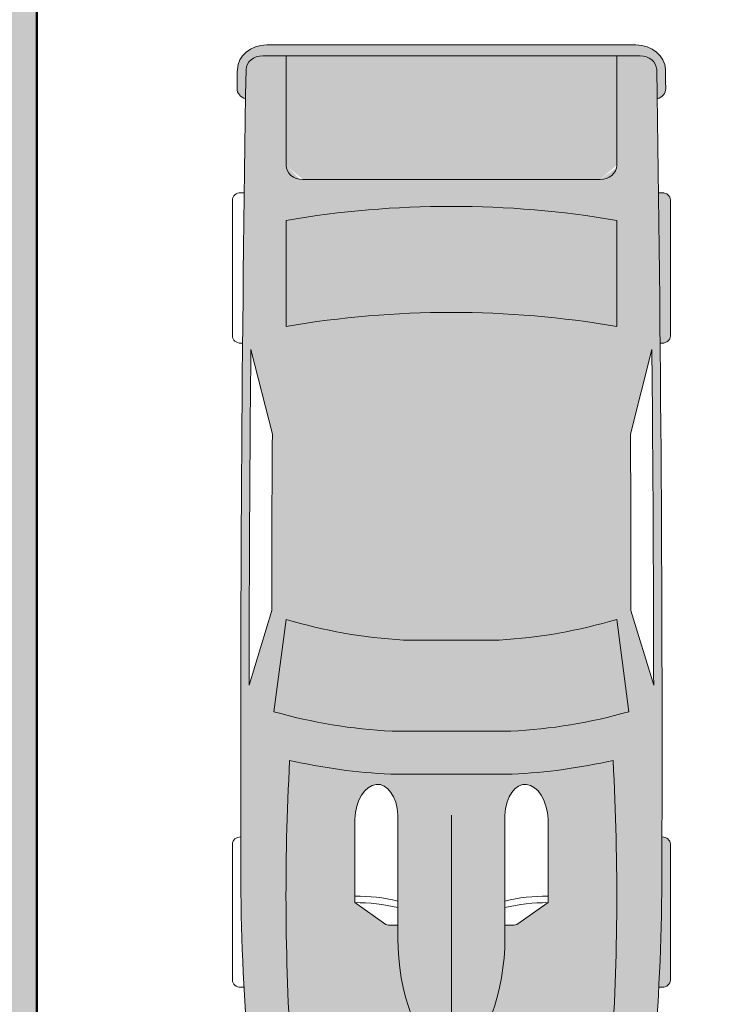
# Model space of a CAD drawing. Units: inches. Extents: x 2419 to 2878, y 1068 to 1713.
# Tile 1 of 20: x 2478 to 2574, y 1153 to 1286. Entities that reach past the tile are written whole.
import ezdxf

# ---------------------------------------------------------------- set-up
doc = ezdxf.new("R2010")
doc.units = ezdxf.units.IN
for name, color, linetype, lineweight in [('A-ANNO-DIMS', 2, 'Continuous', 18), ('A-FLOR-PRKG', 8, 'Continuous', 13), ('A-FLOR-PRKG-PATT', 1, 'Continuous', 13), ('A-FURN-PATT', 254, 'Continuous', 13), ('A-WALL', 7, 'Continuous', 50)]:
    doc.layers.add(name, color=color, linetype=linetype, lineweight=lineweight)
doc.layers.add('A-WALL-PATT', color=18, linetype='Continuous', lineweight=13, true_color=0x000000)
doc.styles.get("Standard").update_dxf_attribs({"font": 'arial.ttf'})
doc.dimstyles.new('ISO-25', dxfattribs={"dimtxt": 12.5, "dimasz": 2.5, "dimexe": 1.25, "dimexo": 0.625, "dimtad": 1, "dimdec": 0, "dimlunit": 4, "dimtxsty": 'Standard', "dimblk": 'ARCHTICK', "dimcen": 2.5, "dimse1": 1, "dimse2": 1, "dimclrd": 4, "dimadec": 0, "dimazin": 0, "dimtfac": 1, "dimtdec": 0, "dimtmove": 0, "dimatfit": 3, "dimfxl": 1, "dimarcsym": 0})

# ---------------------------------------------------------------- blocks, each defined once
blk = doc.blocks.new('*U7')
for p, q in [((46.55368679439944, 38.88847654282876), (22.35054758993934, 38.88847654282876)), ((136.6978032355602, 38.88847654282876), (160.90094244002, 38.88847654282867)), ((21.10406751471477, 37.40863046792069), (21.10406751471477, 36.83230215753705)), ((47.80016686962392, 37.39011648242055), (47.80016686962392, 37.40863046792069)), ((135.4513231603356, 37.07354110333037), (135.4513231603356, 37.40863046792069)), ((162.1474225152445, 37.40863046792049), (162.1474225152445, 36.77402019194128)), ((87.98532186932616, 31.87120872459877), (74.75900729854769, 35.92175679182955)), ((134.313356548143, 35.6043097713567), (119.2882629232503, 31.77757799177584)), ((186.4728846989705, -33.49860931502491), (186.4728846989718, 33.49860931502465)), ((70.0302824853563, 31.53613089391356), (86.40615155322342, 29.35124891408057)), ((188.3990091454065, -32.75868627757393), (188.3990091454077, 32.75868627757058)), ((138.4228833961707, 29.35124891408074), (157.2465674415997, 29.35124891408074)), ((186.4728846989718, 29.35124891408083), (167.0083537481071, 29.35124891408083)), ((164.515393597658, 26.39155676426461), (164.5153935976578, -26.39155676426503)), ((32.26591480791686, 11.62530558863241), (36.12873726252356, 17.16961494239206)), ((36.12873726252356, 17.16961494239206), (50.93891189819171, 17.16961494239206)), ((32.12291633764599, 9.505833383620029), (32.12291633764599, 11.15369945057711)), ((58.9167604809788, -10.77488335095668), (58.9167604809788, 10.77488335095617)), ((66.55009204259746, -10.5288681329018), (66.55009204259746, 10.52886813290129)), ((186.4728846989718, -10.5288681329018), (186.4728846989718, 10.52886813290129)), ((29.77279020470884, 9.505833383620029), (51.68362801571248, 9.505833383620029)), ((82.73706193978568, 8.496039918672748), (82.73706193978568, -8.49603991867258)), ((-4.43e-14, -2.558e-13), (51.68362801571248, -2.558e-13)), ((29.77279020470884, -9.50583338362054), (51.68362801571248, -9.50583338362054)), ((32.12291633764599, -9.50583338362054), (32.12291633764599, -11.15369945057762)), ((32.26591480791686, -11.62530558863292), (36.12873726252356, -17.16961494239257)), ((36.12873726252356, -17.16961494239257), (50.93891189819171, -17.16961494239257)), ((86.40615155322318, -29.35124891408145), (70.03028248535594, -31.53613089391442)), ((157.2465674415997, -29.35124891408117), (138.4228833961707, -29.35124891408126)), ((167.008353748107, -29.35124891408126), (186.4728846989707, -29.35124891408108)), ((87.98532186932607, -31.87120872459903), (74.7590072985476, -35.92175679182964)), ((134.3133565481428, -35.60430977135721), (119.2882629232503, -31.77757799177618)), ((21.10406751471477, -37.4086304679212), (21.10406751471477, -36.83230215753756)), ((47.80016686962392, -37.39011648242107), (47.80016686962392, -37.4086304679212)), ((135.4513231603355, -37.07354110333088), (135.4513231603355, -37.4086304679212)), ((162.1474225152445, -37.408630467921), (162.1474225152445, -36.77402019194179)), ((46.55368679439944, -38.88847654282927), (22.35054758993934, -38.88847654282927)), ((136.6978032355602, -38.88847654282927), (160.9009424400199, -38.88847654282918))]:
    blk.add_line(p, q)
for centre, major_axis, ratio, start_param, end_param in [((22.35054758993934, 37.40863046792072), (2.08e-14, -1.479846074908118), 0.842303869543976, 3.141592653589776, 4.712388980384677), ((46.55368679439944, 37.40863046792072), (2.2e-14, 1.479846074908118), 0.8423038695439758, -1.570796326794884, 1.73e-14), ((136.6978032355602, 37.40863046792072), (2.357e-13, -1.479846074908118), 0.842303869543976, 3.141592653589603, 4.712388980384554), ((160.90094244002, 37.40863046792052), (5.59e-14, 1.479846074908118), 0.842303869543976, -1.570796326794865, 4.44e-14), ((41.19115208863305, -490.8631038926156), (1.294e-13, 528.2339998381949), 0.8423038695439741, 0.0028100083536837, 0.0755983031096952), ((64.48199294511879, -10555.61767587835), (1.907644e-10, 10593.02630634627), 0.842303869543847, -0.0133969486112073, 0.0027970409639888), ((180.6280394947615, 35.8381667808375), (7.4e-14, 2.219769112362114), 0.8423038695439693, -0.0130174256259048, 1.249894140392862), ((64.48199294754608, -10556.35759891604), (1.349839377e-06, 10595.3130398087), 0.8423038681351469, -0.0133969484821159, -0.0130174254969711), ((183.9799245485216, 32.75868627756583), (8.56e-14, -5.246425615115243), 0.8423038695439737, 1.570796326795794, 3.128195704978164), ((64.4819929449925, -10555.61767590795), (1.9177683e-09, -10591.54646030096), 0.8423038695482963, 3.133765086725325, 3.140440689641252), ((183.9799245485226, 33.49860931502124), (3e-16, -2.959692149816168), 0.8423038695439952, 1.570796326796048, 3.128195704978389), ((135.2911776514449, 5.387441675478555), (2.2715e-12, 81.77258453065997), 0.8423038695439563, 1.245306111696802, 1.507880129813836), ((95.78879860270445, -3666.353346297651), (1.949864e-10, -3698.236159209632), 0.8423038695446962, 3.134048706297306, 3.14409775411291), ((37.47375371777758, -593.9621830607928), (6.21e-14, -623.32820996736), 0.8423038695439826, 3.09604606856106, 3.200911180495224), ((134.4003789125686, 5.387441675477674), (4.276e-13, -89.7774543484738), 0.84230386954398, 4.44948196380473, 4.652344057257214), ((149.595361812917, 2.799442537139299), (8.561e-13, -79.57966406425402), 0.842303869543983, 4.372215489277867, 4.640744122441986), ((17.08207736189386, -1.421e-13), (6.87e-14, 147.0179238898305), 0.8423038695439764, 4.511394369635731, 4.913383591133647), ((35.90576140732288, -1.421e-13), (6.87e-14, 147.0179238898305), 0.8423038695439764, 4.511394369635731, 4.913383591133647), ((167.0083537481071, 26.39155676426464), (1.394e-13, 2.959692149816236), 0.842303869543976, 5.55e-14, 1.57079632679492), ((13.03653510440275, 17.00972444508943), (1.2303e-12, 27.41599049210566), 0.8423038695439277, 4.435146050259648, 4.718221029521873), ((14.20086229321332, 17.00972444508943), (1.2303e-12, 27.41599049210566), 0.8423038695439277, 4.435146050259648, 4.718221029521873), ((50.7902773840875, 13.33772416300607), (6.340077547122382, -0.356608581037027), 0.6038335755719145, -1.39555193967809, 1.581314658479915), ((32.74615637525823, 11.15369945057713), (1.313e-13, 0.7399230374541176), 0.8423038695439091, 0.8797135699495516, 1.570796326795045), ((29.77279020470884, -46.66302566589627), (5.12e-14, 56.16885904951626), 0.842303869543976, 7e-16, 0.5903187773915901), ((29.77279020470884, 46.66302566589578), (4.004e-13, 56.16885904951626), 0.8423038695439734, 2.55127387619821, 3.141592653589801), ((149.5953618129329, -2.799442537137565), (4.0897e-12, -79.57966406427697), 0.8423038695439419, -1.499151468852248, -1.230622835688196), ((13.03653510440275, -17.00972444508983), (1.2568e-12, -27.41599049210552), 0.8423038695439318, 1.564964277657711, 1.848039256919935), ((14.20086229321332, -17.00972444508983), (1.2568e-12, -27.41599049210552), 0.8423038695439318, 1.564964277657711, 1.848039256919935), ((32.74615637525823, -11.1536994505777), (1.3e-13, -0.7399230374541176), 0.8423038695439093, 4.712388980384541, 5.403471737230034), ((134.4003789125684, -5.387441675478584), (4.2949e-12, -89.77745434847827), 0.8423038695439354, -1.510751403667474, -1.307889310215002), ((135.2911776514465, -5.387441675480715), (3.2038e-12, -81.77258453066244), 0.8423038695439492, -1.50788012981387, -1.245306111696839), ((167.008353748107, -26.39155676426503), (1.02e-14, -2.959692149816192), 0.8423038695439885, 4.712388980384686, 6.283185307179581), ((37.47375371777847, 593.9621830607904), (1.1693e-12, -623.3282099673584), 0.8423038695439528, -0.0593185269054384, 0.0455465850287298), ((95.78879860271888, 3666.35334629765), (1.637818e-10, -3698.236159209629), 0.8423038695447546, -0.0025051005232382, 0.007543947292366), ((183.9799245485177, -32.7586862775633), (2.428e-13, -5.246425615118353), 0.8423038695439808, 0.0133969486110846, 1.570796326792831), ((183.9799245485216, -33.4986093150211), (9.3e-15, 2.959692149816141), 0.8423038695439732, 3.154989602201626, 4.71238898038339), ((41.19115208863322, 490.8631038926152), (1.37757e-11, -528.2339998381949), 0.8423038695440652, -0.0755983031097181, -0.0028100083537155), ((64.48199294495228, 10555.61767590795), (6.117947e-10, 10593.02630637587), 0.8423038695458146, 3.138795612625926, 3.154989602201039), ((64.48199294503607, 10555.61767590793), (1.6049794e-09, -10591.54646030094), 0.8423038695397146, 0.0011519639481523, 0.0078275668641468), ((180.6280394947581, -35.83816678083949), (2.274e-13, -2.219769112363032), 0.8423038695439803, -1.249894138785958, 0.0130174256254374), ((22.35054758993934, -37.40863046792117), (2.2e-14, 1.479846074908118), 0.8423038695439758, 1.570796326794908, 3.14159265358981), ((46.55368679439944, -37.40863046792117), (2.08e-14, -1.479846074908118), 0.842303869543976, -1.69e-14, 1.570796326794884), ((136.6978032355602, -37.40863046792109), (1.56e-14, -1.479846074908162), 0.8423038695440105, -1.570796326794875, -1.27e-14), ((160.9009424400199, -37.408630467921), (1.969e-13, 1.479846074908162), 0.8423038695440109, 3.141592653589951, 4.712388980384771), ((64.48199294197605, 10556.3575989598), (9.365289701e-07, 10595.31303985772), 0.8423038705260315, 3.154610079306566, 3.154989602290631)]:
    blk.add_ellipse(centre, major_axis=major_axis, ratio=ratio, start_param=start_param, end_param=end_param)
at = {"extrusion": (0, 0, -1)}
blk.add_ellipse((50.7902773840875, -13.33772416300655), major_axis=(6.340077547122382, 0.3566085810370246), ratio=0.6038335755719145, start_param=-1.39555193967809, end_param=1.581314658479915, dxfattribs=at)
blk = doc.blocks.new('_ArchTick')
at = {"color": 0, "linetype": 'ByBlock', "const_width": 0.15}
blk.add_lwpolyline([(-0.5, -0.5), (0.5, 0.5)], dxfattribs=at)
blk = doc.blocks.new('*D38')
at = {"layer": 'A-ANNO-DIMS', "color": 4, "lineweight": -2, "transparency": 16777216}
for p, q in [((2444.314464000002, 1165.602617), (2444.314464000002, 1212.505754789905)), ((2444.314464000002, 1130.812987), (2444.314464000002, 1165.602617))]:
    blk.add_line(p, q, dxfattribs=at)
at = {"layer": 'Defpoints', "color": 0, "transparency": 16777216}
for p in [(2444.314464000002, 1165.602617), (2656.740829000001, 1165.602617), (2656.740829000001, 1130.812987)]:
    blk.add_point(p, dxfattribs=at)
at = {"layer": 'A-ANNO-DIMS', "color": 4, "lineweight": -2, "transparency": 16777216, "xscale": 2.5, "yscale": 2.5, "zscale": 2.5}
for p, rotation in [((2444.314464000002, 1165.602617), 90), ((2444.314464000002, 1130.812987), 270)]:
    blk.add_blockref('_ArchTick', p, dxfattribs=dict(at, rotation=rotation))
at = {"layer": 'A-ANNO-DIMS', "color": 0, "transparency": 16777216, "insert": (2437.413884190998, 1190.304185894951), "char_height": 12.5, "attachment_point": 5, "rotation": 90}
blk.add_mtext('2\'-11"', dxfattribs=at)
blk = doc.blocks.new('*D43')
at = {"layer": 'A-ANNO-DIMS', "color": 4, "lineweight": -2, "transparency": 16777216}
blk.add_line((2480.514464, 1079.924615), (2557.299401, 1079.924615), dxfattribs=at)
at = {"layer": 'Defpoints', "color": 0, "transparency": 16777216}
for p in [(2480.514464, 1408.812987), (2557.299401, 1408.812987), (2557.299401, 1079.924615)]:
    blk.add_point(p, dxfattribs=at)
at = {"layer": 'A-ANNO-DIMS', "color": 4, "lineweight": -2, "transparency": 16777216, "xscale": 2.5, "yscale": 2.5, "zscale": 2.5, "rotation": 180}
blk.add_blockref('_ArchTick', (2480.514464, 1079.924615), dxfattribs=at)
at = {"layer": 'A-ANNO-DIMS', "color": 4, "lineweight": -2, "transparency": 16777216, "xscale": 2.5, "yscale": 2.5, "zscale": 2.5}
blk.add_blockref('_ArchTick', (2557.299401, 1079.924615), dxfattribs=at)
at = {"layer": 'A-ANNO-DIMS', "color": 0, "transparency": 16777216, "insert": (2518.9069325, 1086.931777346521), "char_height": 12.5, "attachment_point": 5}
blk.add_mtext('6\'-5"', dxfattribs=at)
blk = doc.blocks.new('*D44')
at = {"layer": 'A-ANNO-DIMS', "color": 4, "lineweight": -2, "transparency": 16777216}
for p, q in [((2557.299401, 1079.924615), (2585.817994, 1079.924615)), ((2585.817994, 1079.924615), (2652.136206824011, 1079.924615))]:
    blk.add_line(p, q, dxfattribs=at)
at = {"layer": 'Defpoints', "color": 0, "transparency": 16777216}
for p in [(2557.299401, 1408.812987), (2585.817994, 1408.812987), (2585.817994, 1079.924615)]:
    blk.add_point(p, dxfattribs=at)
at = {"layer": 'A-ANNO-DIMS', "color": 4, "lineweight": -2, "transparency": 16777216, "xscale": 2.5, "yscale": 2.5, "zscale": 2.5, "rotation": 180}
blk.add_blockref('_ArchTick', (2557.299401, 1079.924615), dxfattribs=at)
at = {"layer": 'A-ANNO-DIMS', "color": 4, "lineweight": -2, "transparency": 16777216, "xscale": 2.5, "yscale": 2.5, "zscale": 2.5}
blk.add_blockref('_ArchTick', (2585.817994, 1079.924615), dxfattribs=at)
at = {"layer": 'A-ANNO-DIMS', "color": 0, "transparency": 16777216, "insert": (2620.227100412006, 1087.012780075034), "char_height": 12.5, "attachment_point": 5}
blk.add_mtext('2\'-4 1/2"', dxfattribs=at)
blk = doc.blocks.new('*D54')
at = {"layer": 'A-ANNO-DIMS', "color": 4, "lineweight": -2, "transparency": 16777216}
blk.add_line((2444.314464000002, 1130.812987), (2444.314464000002, 1293.812987), dxfattribs=at)
at = {"layer": 'Defpoints', "color": 0, "transparency": 16777216}
for p in [(2444.314464000002, 1293.812987), (2480.514464000001, 1293.812987), (2480.514464000001, 1130.812987)]:
    blk.add_point(p, dxfattribs=at)
at = {"layer": 'A-ANNO-DIMS', "color": 4, "lineweight": -2, "transparency": 16777216, "xscale": 2.5, "yscale": 2.5, "zscale": 2.5}
for p, rotation in [((2444.314464000002, 1293.812987), 90), ((2444.314464000002, 1130.812987), 270)]:
    blk.add_blockref('_ArchTick', p, dxfattribs=dict(at, rotation=rotation))
at = {"layer": 'A-ANNO-DIMS', "color": 0, "transparency": 16777216, "insert": (2437.30303835198, 1212.312987), "char_height": 12.5, "attachment_point": 5, "rotation": 90}
blk.add_mtext('13\'-7"', dxfattribs=at)
blk = doc.blocks.new('*D56')
at = {"layer": 'A-ANNO-DIMS', "color": 4, "lineweight": -2, "transparency": 16777216}
for p, q in [((2480.514464, 1079.924615), (2503.967101000001, 1079.924615)), ((2503.967101000001, 1079.924615), (2578.607278353343, 1079.924615))]:
    blk.add_line(p, q, dxfattribs=at)
at = {"layer": 'Defpoints', "color": 0, "transparency": 16777216}
for p in [(2480.514464, 1507.812987), (2503.967101000001, 1494.852151), (2503.967101000001, 1079.924615)]:
    blk.add_point(p, dxfattribs=at)
at = {"layer": 'A-ANNO-DIMS', "color": 4, "lineweight": -2, "transparency": 16777216, "xscale": 2.5, "yscale": 2.5, "zscale": 2.5, "rotation": 180}
blk.add_blockref('_ArchTick', (2480.514464, 1079.924615), dxfattribs=at)
at = {"layer": 'A-ANNO-DIMS', "color": 4, "lineweight": -2, "transparency": 16777216, "xscale": 2.5, "yscale": 2.5, "zscale": 2.5}
blk.add_blockref('_ArchTick', (2503.967101000001, 1079.924615), dxfattribs=at)
at = {"layer": 'A-ANNO-DIMS', "color": 0, "transparency": 16777216, "insert": (2542.537189676672, 1087.012780075034), "char_height": 12.5, "attachment_point": 5}
blk.add_mtext('1\'-11 1/2"', dxfattribs=at)
blk = doc.blocks.new('*D59')
at = {"layer": 'A-ANNO-DIMS', "color": 4, "lineweight": -2, "transparency": 16777216}
blk.add_line((2480.514464, 1079.924615), (2589.514464, 1079.924615), dxfattribs=at)
at = {"layer": 'Defpoints', "color": 0, "transparency": 16777216}
for p in [(2480.514464, 1414.812987), (2589.514464, 1414.812987), (2589.514464, 1079.924615)]:
    blk.add_point(p, dxfattribs=at)
at = {"layer": 'A-ANNO-DIMS', "color": 4, "lineweight": -2, "transparency": 16777216, "xscale": 2.5, "yscale": 2.5, "zscale": 2.5, "rotation": 180}
blk.add_blockref('_ArchTick', (2480.514464, 1079.924615), dxfattribs=at)
at = {"layer": 'A-ANNO-DIMS', "color": 4, "lineweight": -2, "transparency": 16777216, "xscale": 2.5, "yscale": 2.5, "zscale": 2.5}
blk.add_blockref('_ArchTick', (2589.514464, 1079.924615), dxfattribs=at)
at = {"layer": 'A-ANNO-DIMS', "color": 0, "transparency": 16777216, "insert": (2535.014464, 1086.931777346521), "char_height": 12.5, "attachment_point": 5}
blk.add_mtext('9\'-1"', dxfattribs=at)

msp = doc.modelspace()

# ---------------------------------------------------------------- hatches: boundary and pattern name
at = {"layer": 'A-FLOR-PRKG-PATT'}
h = msp.add_hatch(color=256, dxfattribs=at)
h.dxf.hatch_style = 1
edge = h.paths.add_edge_path()
edge.add_ellipse((2561.373836383861, 1279.453459119739), major_axis=(3.988072461255025, 3.66e-13), ratio=0.8423038695438922, start_angle=0.6465540970538215, end_angle=89.99999999985512)
edge.add_line((2561.373836383866, 1282.812627985876), (2511.5707802864, 1282.812627985877))
edge.add_ellipse((2511.570780286403, 1279.453459119742), major_axis=(3.98807246125278, 1.3091e-12), ratio=0.8423038695439103, start_angle=90.00000000004323, end_angle=179.3534459029021)
edge.add_ellipse((10560.89162156784, 1188.617060177679), major_axis=(-8054.031306696497, 2.4305759344e-06), ratio=0.8423038662355361, start_angle=-0.6465540797578173, end_angle=-0.6282371989246356)
edge.add_ellipse((2509.229911990343, 1276.90552239923), major_axis=(1.687358349624694, 2.5733e-12), ratio=0.8423038695439247, start_angle=179.3717627837196, end_angle=248.4647566009239)
edge.add_ellipse((10560.32916878445, 1188.617060175834), major_axis=(8052.293045373481, 7.264082e-10), ratio=0.842303869546111, start_angle=179.353445902933, end_angle=179.3813568036757, ccw=False)
edge.add_ellipse((2511.008327503194, 1279.453459119743), major_axis=(2.249811132832755, 8.714e-13), ratio=0.842303869544046, start_angle=90.0000000000465, end_angle=179.353445902909, ccw=False)
edge.add_line((2511.008327503191, 1281.348483742671), (2561.936289167075, 1281.34848374267))
edge.add_ellipse((2561.936289167072, 1279.453459119742), major_axis=(-2.249811132833226, 1.1022e-12), ratio=0.8423038695438698, start_angle=180.64655409712, end_angle=269.99999999993184, ccw=False)
edge.add_ellipse((-5487.384552136685, 1188.617060175704), major_axis=(8052.293045395979, 3.62524e-11), ratio=0.8423038695435844, start_angle=0.5282714718171064, end_angle=0.6465540970606867, ccw=False)
edge.add_ellipse((2563.714704679924, 1276.905522399228), major_axis=(-1.687358349625589, 1.0166e-12), ratio=0.8423038695437657, start_angle=111.5352435040611, end_angle=180.6282372162117)
edge.add_ellipse((-5487.947004930842, 1188.617060173442), major_axis=(-8054.031306737888, 1.1179418355e-06), ratio=0.8423038710930354, start_angle=180.628237224196, end_angle=180.6465541050291)
edge = h.paths.add_edge_path()
edge.add_ellipse((2564.908493259296, 1261.909961940352), major_axis=(-1.1249055664166, 6.787e-13), ratio=0.8423038695440812, start_angle=180.0000000000345, end_angle=270.0000000000346)
edge.add_line((2564.908493259296, 1262.857474251817), (2564.426094012466, 1262.857474251817))
edge.add_ellipse((-5487.384552136685, 1188.617060175704), major_axis=(8052.293045395979, 3.62524e-11), ratio=0.8423038695435844, start_angle=0.38386677879208264, end_angle=0.5282714718171064, ccw=False)
edge.add_line((2564.653774949148, 1242.564423998052), (2564.908493259296, 1242.564423998052))
edge.add_ellipse((2564.908493259296, 1243.511936309516), major_axis=(-1.1249055664166, 1.035e-13), ratio=0.8423038695438789, start_angle=90.00000000000524, end_angle=180.0000000000052)
edge.add_line((2566.033398825713, 1243.511936309516), (2566.033398825713, 1261.909961940352))
edge = h.paths.add_edge_path()
edge.add_ellipse((2564.908493259296, 1174.988851318627), major_axis=(1.1249055664166, 1.037e-13), ratio=0.8423038695438791, start_angle=-5.283e-12, end_angle=89.99999999999471)
edge.add_line((2564.908493259296, 1175.936363630091), (2564.894419846052, 1175.936363630091))
edge.add_ellipse((-5487.384552136685, 1188.617060175704), major_axis=(8052.293045395979, 3.62524e-11), ratio=0.8423038695435844, start_angle=-0.13498657685727267, end_angle=-0.0902290885933894, ccw=False)
edge.add_ellipse((2163.342529988697, 1170.912518487192), major_axis=(401.5372793588411, 5.38767e-11), ratio=0.8423038695443597, start_angle=-2.1799503136529097, end_angle=-0.13561239044622653, ccw=False)
edge.add_line((2564.470397071167, 1155.643313376326), (2564.908493259296, 1155.643313376326))
edge.add_ellipse((2564.908493259296, 1156.59082568779), major_axis=(-1.1249055664166, 1.035e-13), ratio=0.8423038695438789, start_angle=90.00000000000524, end_angle=180.0000000000052)
edge.add_line((2566.033398825713, 1156.59082568779), (2566.033398825713, 1174.988851318627))
h.paths.add_polyline_path([(2574.475657961183, 1207.447993793836), (2633.939672590987, 1207.447993793836), (2633.939672590987, 1217.366392668578), (2574.475657961183, 1217.366392668578)], flags=9)
h.paths.add_polyline_path([(2574.453572904682, 1217.827970349456), (2610.472091552684, 1217.827970349456), (2610.472091552684, 1227.878879563206), (2574.453572904682, 1227.878879563206)], flags=9)
h.paths.add_polyline_path([(2672.426489674963, 1304.020425493039), (2718.617385347474, 1304.020425493039), (2718.617385347474, 1313.938824367782), (2672.426489674963, 1313.938824367782)], flags=9)
h.paths.add_polyline_path([(2672.404404618462, 1314.40040204866), (2750.128343963557, 1314.40040204866), (2750.128343963557, 1324.45131126241), (2672.404404618462, 1324.45131126241)], flags=9)
h.paths.add_polyline_path([(2500.431978237712, 1374.443618551611), (2544.803065254515, 1374.443618551611), (2544.803065254515, 1384.362017426354), (2500.431978237712, 1384.362017426354)], flags=9)
h.paths.add_polyline_path([(2500.409893181211, 1384.823595107232), (2566.075391676585, 1384.823595107232), (2566.075391676585, 1394.874504320982), (2500.409893181211, 1394.874504320982)], flags=9)
h.paths.add_polyline_path([(2738.933372766964, 1376.749079437844), (2778.273483912766, 1376.749079437844), (2778.273483912766, 1386.667478312586), (2738.933372766964, 1386.667478312586)], flags=9)
h.paths.add_polyline_path([(2659.120436878741, 1357.799561515192), (2703.491523895543, 1357.799561515192), (2703.491523895543, 1367.717960389935), (2659.120436878741, 1367.717960389935)], flags=9)
h.paths.add_polyline_path([(2659.09835182224, 1368.179538070813), (2694.114208905082, 1368.179538070813), (2694.114208905082, 1378.230447284563), (2659.09835182224, 1378.230447284563)], flags=9)
h.paths.add_polyline_path([(2730.122846517376, 1466.067315328676), (2769.462957663177, 1466.067315328676), (2769.462957663177, 1475.985714203419), (2730.122846517376, 1475.985714203419)], flags=9)
h.paths.add_polyline_path([(2730.100761460875, 1476.447291884297), (2765.116618543717, 1476.447291884297), (2765.116618543717, 1486.498201098047), (2730.100761460875, 1486.498201098047)], flags=9)
h.paths.add_polyline_path([(2730.381989889755, 1518.64710392716), (2761.479957949264, 1518.64710392716), (2761.479957949264, 1528.565502801902), (2730.381989889755, 1528.565502801902)], flags=9)
h.paths.add_polyline_path([(2730.361009086079, 1529.028184735605), (2780.957873530603, 1529.028184735605), (2780.957873530603, 1539.072468432406), (2730.361009086079, 1539.072468432406)], flags=9)
h.paths.add_polyline_path([(2629.32015605144, 1455.188736350721), (2688.784170681244, 1455.188736350721), (2688.784170681244, 1465.107135225464), (2629.32015605144, 1465.107135225464)], flags=9)
h.paths.add_polyline_path([(2629.298070994938, 1465.568712906342), (2681.902467075432, 1465.568712906342), (2681.902467075432, 1475.619622120092), (2629.298070994938, 1475.619622120092)], flags=9)
h.paths.add_polyline_path([(2513.228616334912, 1456.483806675948), (2562.630679222714, 1456.483806675948), (2562.630679222714, 1466.402205550691), (2513.228616334912, 1466.402205550691)], flags=9)
h.paths.add_polyline_path([(2513.207635531236, 1466.864887484394), (2556.260244674908, 1466.864887484394), (2556.260244674908, 1476.909171181194), (2513.207635531236, 1476.909171181194)], flags=9)
h.paths.add_polyline_path([(2488.870122348878, 1521.537768100923), (2519.968090408386, 1521.537768100923), (2519.968090408386, 1531.456166975666), (2488.870122348878, 1531.456166975666)], flags=9)
h.paths.add_polyline_path([(2536.549469908388, 1543.50690417551), (2580.92276543084, 1543.50690417551), (2580.92276543084, 1553.431928567203), (2536.549469908388, 1553.431928567203)], flags=9)
h.paths.add_polyline_path([(2536.557199678163, 1553.921112568707), (2573.525375755723, 1553.921112568707), (2573.525375755723, 1563.799758341748), (2536.557199678163, 1563.799758341748)], flags=9)
h = msp.add_hatch(color=256, dxfattribs=at)
h.dxf.hatch_style = 1
edge = h.paths.add_edge_path(flags=17)
edge.add_line((2558.78367155362, 1281.34848374267), (2514.160945116646, 1281.348483742671))
edge.add_line((2514.160945116646, 1281.348483742671), (2514.160945116646, 1266.552513009246))
edge.add_ellipse((2516.410756249479, 1266.552513009246), major_axis=(2.249811132832746, 7.445e-13), ratio=0.8423038695441503, start_angle=179.999999999981, end_angle=269.999999999981)
edge.add_line((2516.410756249479, 1264.657488386317), (2556.533860420787, 1264.657488386317))
edge.add_ellipse((2556.533860420787, 1266.552513009246), major_axis=(2.249811132833201, 8.993e-13), ratio=0.8423038695438791, start_angle=269.9999999999771, end_angle=359.9999999999771)
edge.add_line((2558.78367155362, 1266.552513009246), (2558.78367155362, 1281.34848374267))
edge = h.paths.add_edge_path()
edge.add_ellipse((-5487.384552136685, 1188.617060175704), major_axis=(8052.293045395979, 3.62524e-11), ratio=0.8423038695435844, start_angle=0.3838667787920817, end_angle=0.5282714718171219)
edge.add_ellipse((-5487.384552136685, 1188.617060175704), major_axis=(8052.293045395979, 3.62524e-11), ratio=0.8423038695435844, start_angle=0.5282714718171219, end_angle=0.6465540970607009)
edge.add_ellipse((2561.936289167072, 1279.453459119742), major_axis=(-2.249811132833226, 1.1022e-12), ratio=0.8423038695438698, start_angle=180.6465540971199, end_angle=269.9999999999318)
edge.add_line((2561.936289167075, 1281.34848374267), (2558.78367155362, 1281.34848374267))
edge.add_line((2558.78367155362, 1281.34848374267), (2558.78367155362, 1266.266612494733))
edge.add_ellipse((2556.533860420787, 1266.552513009246), major_axis=(2.249811132833201, 8.993e-13), ratio=0.8423038695438791, start_angle=269.9999999999771, end_angle=359.9999999999771, ccw=False)
edge.add_line((2556.533860420787, 1264.657488386317), (2516.071329440636, 1264.657488386317))
edge.add_ellipse((2516.410756249479, 1266.552513009246), major_axis=(2.249811132832746, 7.445e-13), ratio=0.8423038695441503, start_angle=179.9999999999811, end_angle=269.999999999981, ccw=False)
edge.add_line((2514.160945116646, 1266.552513009246), (2514.160945116646, 1281.348483742671))
edge.add_line((2514.160945116646, 1281.348483742671), (2511.008327503191, 1281.348483742671))
edge.add_ellipse((2511.008327503194, 1279.453459119743), major_axis=(2.249811132832755, 8.714e-13), ratio=0.842303869544046, start_angle=90.00000000004655, end_angle=179.3534459029089)
edge.add_ellipse((10560.32916878445, 1188.617060175834), major_axis=(8052.293045373481, 7.264082e-10), ratio=0.842303869546111, start_angle=179.3534459029329, end_angle=179.3813568036756)
edge.add_ellipse((10560.32916878445, 1188.617060175834), major_axis=(8052.293045373481, 7.264082e-10), ratio=0.842303869546111, start_angle=179.3813568036756, end_angle=179.4717285281769)
edge.add_ellipse((10560.32916878445, 1188.617060175834), major_axis=(8052.293045373481, 7.264082e-10), ratio=0.842303869546111, start_angle=179.4717285281769, end_angle=179.6161332212023)
edge.add_ellipse((10560.32916878445, 1188.617060175834), major_axis=(8052.293045373481, 7.264082e-10), ratio=0.842303869546111, start_angle=179.6161332212023, end_angle=180.0902290885891)
edge.add_ellipse((10560.32916878445, 1188.617060175834), major_axis=(8052.293045373481, 7.264082e-10), ratio=0.842303869546111, start_angle=180.0902290885891, end_angle=180.1349865768531)
edge.add_ellipse((2909.602086681569, 1170.912518487192), major_axis=(401.537279358841, 1.00104e-11), ratio=0.8423038695439784, start_angle=180.1806905311021, end_angle=182.1799503136438)
edge.add_ellipse((2909.602086681569, 1170.912518487192), major_axis=(401.537279358841, 1.00104e-11), ratio=0.8423038695439784, start_angle=182.1799503136438, end_angle=183.6504275856975)
edge.add_ellipse((2557.395012080375, 1341.823872000969), major_axis=(238.1610159604077, 8.386761e-10), ratio=0.8423038695464203, start_angle=256.2194710103002, end_angle=257.874034447514)
edge.add_ellipse((2987.972891601874, 1168.086736677267), major_axis=(-473.8231799819343, 8.8666e-12), ratio=0.8423038695441055, start_angle=-2.19854056595409, end_angle=2.8637146078386877, ccw=False)
edge.add_ellipse((2532.377042461035, 1241.765548321486), major_axis=(-68.24436665927666, 5.9291e-12), ratio=0.8423038695438547, start_angle=72.28004677725448, end_angle=85.9175893088543)
edge.add_line((2528.281776586936, 1184.386646564943), (2544.66284008333, 1184.386646564943))
edge.add_ellipse((2540.567574209232, 1241.765548321486), major_axis=(68.24436665927627, 7.0353e-12), ratio=0.8423038695438563, start_angle=-85.91758930885564, end_angle=-72.28004677725573)
edge.add_ellipse((2084.971725068394, 1168.086736677268), major_axis=(473.8231799819329, 7.7093e-12), ratio=0.842303869544119, start_angle=-2.863714607838574, end_angle=2.19854056595409, ccw=False)
edge.add_ellipse((2515.549604589891, 1341.823872000969), major_axis=(238.1610159617672, 7.268827e-10), ratio=0.8423038695418011, start_angle=-77.87403444789076, end_angle=-76.21947101067707)
edge.add_ellipse((2163.342529988697, 1170.912518487192), major_axis=(401.5372793588411, 5.38767e-11), ratio=0.8423038695443597, start_angle=-3.650427585706752, end_angle=-2.179950313652928)
edge.add_ellipse((2163.342529988697, 1170.912518487192), major_axis=(401.5372793588411, 5.38767e-11), ratio=0.8423038695443597, start_angle=-2.179950313652928, end_angle=-0.1356123904461693)
edge.add_ellipse((-5487.384552136685, 1188.617060175704), major_axis=(8052.293045395979, 3.62524e-11), ratio=0.8423038695435844, start_angle=-0.1349865768572857, end_angle=-0.0902290885934275)
edge.add_ellipse((-5487.384552136685, 1188.617060175704), major_axis=(8052.293045395979, 3.62524e-11), ratio=0.8423038695435844, start_angle=-0.0902290885934275, end_angle=0.3838667787920817)
edge = h.paths.add_edge_path(flags=16)
edge.add_ellipse((2538.600305662885, 1253.316020452369), major_axis=(-60.4925124290502, 2.2066e-12), ratio=0.8423038695439758, start_angle=94.87006959713776, end_angle=112.7919148775885)
edge.add_line((2558.78367155362, 1205.282717824576), (2560.444510435955, 1192.834594616562))
edge.add_ellipse((2540.567574209233, 1242.442689327507), major_axis=(62.15946177006578, 2.00584e-11), ratio=0.8423038695437449, start_angle=-85.72257903696442, end_angle=-68.16504620330988, ccw=False)
edge.add_line((2544.475831520138, 1190.18912650496), (2528.468785150127, 1190.18912650496))
edge.add_ellipse((2532.377042461034, 1242.442689327506), major_axis=(-62.15946177005032, 4.9036e-12), ratio=0.8423038695439334, start_angle=68.16504620329499, end_angle=85.72257903694901, ccw=False)
edge.add_line((2512.500106234312, 1192.834594616562), (2514.160945116646, 1205.282717824576))
edge.add_ellipse((2534.344311007379, 1253.316020452358), major_axis=(60.49251242903284, 5.7929e-12), ratio=0.8423038695440167, start_angle=247.2080851224046, end_angle=265.1299304028586)
edge.add_line((2530.014040303706, 1202.493657935295), (2542.93057636656, 1202.493657935295))
edge = h.paths.add_edge_path(flags=16)
edge.add_ellipse((-250.5076064213731, 1212.41494060954), major_axis=(2811.215647327496, 7.69506e-11), ratio=0.8423038695473968, start_angle=-0.1208973690345315, end_angle=0.3640763488885457)
edge.add_line((2560.628046540813, 1230.278067505092), (2563.536938183683, 1241.699398237495))
edge.add_ellipse((-5487.384552136674, 1188.617060175768), major_axis=(8051.168139829552, 1.0212802e-09), ratio=0.8423038695408568, start_angle=0.05559431349178112, end_angle=0.3777641939024079, ccw=False)
edge.add_line((2563.77824565912, 1196.42913661293), (2560.699219978594, 1206.483124751376))
edge = h.paths.add_edge_path(flags=16)
edge.add_ellipse((2536.472308335133, 1152.58599600549), major_axis=(111.7557317283417, 6.024e-13), ratio=0.8423038695439972, start_angle=76.40186530976897, end_angle=103.5981346902301)
edge.add_line((2514.160945116646, 1244.823256661064), (2514.160945116646, 1259.132087371369))
edge.add_ellipse((2536.472308335133, 1166.894826715795), major_axis=(111.7557317283482, 6.52e-13), ratio=0.8423038695439483, start_angle=76.401865309769, end_angle=103.5981346902301, ccw=False)
edge.add_line((2558.78367155362, 1259.13208737137), (2558.78367155362, 1244.823256661064))
edge = h.paths.add_edge_path(flags=16)
edge.add_line((2512.24539669167, 1206.483124751367), (2509.166371011145, 1196.429136612926))
edge.add_ellipse((10560.32916880695, 1188.617060175738), major_axis=(8051.168139829567, 3.955788e-10), ratio=0.8423038695452166, start_angle=179.6222358060874, end_angle=179.9444056864979, ccw=False)
edge.add_line((2509.407678486582, 1241.699398237499), (2512.316570129453, 1230.278067505094))
edge.add_ellipse((5323.452223091639, 1212.41494060953), major_axis=(2811.215647327498, 3.441147e-10), ratio=0.8423038695471676, start_angle=179.6359236511027, end_angle=180.1208973690256)
edge = h.paths.add_edge_path()
edge.add_ellipse((2084.971725068394, 1168.086736677268), major_axis=(473.8231799819329, 7.7093e-12), ratio=0.842303869544119, start_angle=-2.863714607838618, end_angle=2.198540565954143)
edge.add_ellipse((2540.567574209232, 1241.765548321486), major_axis=(68.24436665927627, 7.0353e-12), ratio=0.8423038695438563, start_angle=-85.91758930885561, end_angle=-72.28004677725562, ccw=False)
edge.add_line((2544.66284008333, 1184.386646564943), (2528.281776586936, 1184.386646564943))
edge.add_ellipse((2532.377042461035, 1241.765548321486), major_axis=(-68.24436665927666, 5.9291e-12), ratio=0.8423038695438547, start_angle=72.28004677725448, end_angle=85.91758930885442, ccw=False)
edge.add_ellipse((2987.972891601874, 1168.086736677267), major_axis=(-473.8231799819343, 8.8666e-12), ratio=0.8423038695441055, start_angle=-2.198540565954097, end_angle=2.86371460783868)
edge.add_ellipse((2557.395012080375, 1336.613039816894), major_axis=(232.0761110713879, 4.935805e-10), ratio=0.8423038695458167, start_angle=257.5553727064329, end_angle=259.7904610027336)
edge.add_ellipse((2496.642822767904, 984.1543496287911), major_axis=(190.7675054597987, 1.126016e-10), ratio=0.8423038695444711, start_angle=77.44506735582888, end_angle=80.7434339927645, ccw=False)
edge.add_line((2531.813886249475, 1142.084050780911), (2536.163633413452, 1139.678766703385))
edge.add_ellipse((2536.472308335133, 1140.07480444526), major_axis=(-0.5624527832082081, 2e-16), ratio=0.8423038695442194, start_angle=52.06686954015882, end_angle=90.00000000000001)
edge.add_line((2536.472308335133, 1139.601048289528), (2536.472308335133, 1142.214540749464))
edge.add_ellipse((2571.943225349704, 1162.232846283187), major_axis=(42.69677993908317, 2.1357e-12), ratio=0.8423038695439387, start_angle=179.9999999999972, end_angle=209.4385695979767, ccw=False)
edge.add_line((2529.246445410621, 1162.232846283187), (2529.246445410621, 1164.019295572439))
edge.add_line((2529.246445410621, 1164.019295572439), (2527.791345403533, 1164.019295572439))
edge.add_line((2527.791345403533, 1164.019295572439), (2523.420818893486, 1167.064321898398))
edge.add_line((2523.420818893486, 1167.064321898398), (2523.420818893486, 1178.322281877985))
edge.add_ellipse((2526.333632152054, 1178.20929729458), major_axis=(0.2710761508483066, 4.819412400518167), ratio=0.6038335755720334, start_angle=-73.65740804575063, end_angle=90.99798572492182, ccw=False)
edge.add_line((2529.246445410621, 1178.88837812286), (2529.246445410621, 1162.232846283187))
edge.add_ellipse((2571.943225349704, 1162.232846283187), major_axis=(42.69677993908317, 2.1357e-12), ratio=0.8423038695439387, start_angle=179.9999999999971, end_angle=209.4385695979767)
edge.add_ellipse((2501.001391320562, 1162.232846283187), major_axis=(42.69677993908317, 6.184e-12), ratio=0.8423038695440235, start_angle=-29.43856959798787, end_angle=-8.2942e-12)
edge.add_line((2543.698171259645, 1162.232846283187), (2543.698171259645, 1178.88837812286))
edge.add_ellipse((2546.610984518212, 1178.20929729458), major_axis=(-0.2710761508525395, 4.819412400518348), ratio=0.6038335755718809, start_angle=269.00201427502856, end_angle=433.65740804570055, ccw=False)
edge.add_line((2549.52379777678, 1178.322281877985), (2549.52379777678, 1167.064321898398))
edge.add_line((2549.52379777678, 1167.064321898398), (2545.153271266734, 1164.019295572439))
edge.add_line((2545.153271266734, 1164.019295572439), (2543.698171259645, 1164.019295572439))
edge.add_line((2543.698171259645, 1164.019295572439), (2543.698171259645, 1162.232846283187))
edge.add_ellipse((2501.001391320562, 1162.232846283187), major_axis=(42.69677993908317, 6.184e-12), ratio=0.8423038695440235, start_angle=-29.438569597987794, end_angle=-8.29913915367797e-12, ccw=False)
edge.add_line((2536.472308335133, 1142.214540749463), (2536.472308335133, 1139.601048289528))
edge.add_ellipse((2536.472308335133, 1140.07480444526), major_axis=(-0.5624527832082081, 2e-16), ratio=0.8423038695442194, start_angle=90.00000000000001, end_angle=127.9331304598412)
edge.add_line((2536.780983256814, 1139.678766703385), (2541.130730420792, 1142.084050780911))
edge.add_ellipse((2576.301793902363, 984.1543496287911), major_axis=(190.767505459939, 3.39412e-11), ratio=0.8423038695438718, start_angle=99.25656600719128, end_angle=102.55493264412712, ccw=False)
edge.add_ellipse((2515.549604589896, 1336.613039816892), major_axis=(-232.0761110718477, 5.10817e-11), ratio=0.8423038695441782, start_angle=100.2095389971557, end_angle=102.4446272934566)
at = {"layer": 'A-FURN-PATT'}
h = msp.add_hatch(color=256, dxfattribs=at)
h.dxf.hatch_style = 1
h.paths.add_polyline_path([(2693.678900285153, 1539.212987234935), (2678.478910285153, 1539.212987234935), (2678.478910285153, 1552.012987234935), (2633.678910285153, 1552.012987234935), (2633.678910285153, 1488.812957234935), (2693.678900285153, 1488.812957234935)])
edge = h.paths.add_edge_path()
edge.add_ellipse((2538.600305662885, 1253.316020452369), major_axis=(-60.4925124290502, 2.2066e-12), ratio=0.8423038695439758, start_angle=94.87006959713779, end_angle=112.7919148775886, ccw=False)
edge.add_line((2542.930576366559, 1202.493657935295), (2530.014040303706, 1202.493657935295))
edge.add_ellipse((2534.344311007379, 1253.316020452358), major_axis=(60.49251242903284, 5.7929e-12), ratio=0.8423038695440167, start_angle=247.2080851224046, end_angle=265.1299304028586, ccw=False)
edge.add_line((2514.160945116646, 1205.282717824576), (2512.500106234312, 1192.834594616562))
edge.add_ellipse((2532.377042461034, 1242.442689327506), major_axis=(-62.15946177005032, 4.9036e-12), ratio=0.8423038695439334, start_angle=68.16504620329505, end_angle=85.72257903694899)
edge.add_line((2528.468785150127, 1190.18912650496), (2544.475831520138, 1190.18912650496))
edge.add_ellipse((2540.567574209233, 1242.442689327507), major_axis=(62.15946177006578, 2.00584e-11), ratio=0.8423038695437449, start_angle=-85.72257903696453, end_angle=-68.16504620331001)
edge.add_line((2560.444510435955, 1192.834594616562), (2558.78367155362, 1205.282717824576))
edge = h.paths.add_edge_path()
edge.add_ellipse((2536.472308335133, 1166.894826715795), major_axis=(111.7557317283482, 6.52e-13), ratio=0.8423038695439483, start_angle=76.40186530976897, end_angle=103.5981346902301)
edge.add_line((2514.160945116646, 1259.132087371369), (2514.160945116646, 1244.823256661064))
edge.add_ellipse((2536.472308335133, 1152.58599600549), major_axis=(111.7557317283417, 6.024e-13), ratio=0.8423038695439972, start_angle=76.401865309769, end_angle=103.59813469023021, ccw=False)
edge.add_line((2558.78367155362, 1244.823256661064), (2558.78367155362, 1259.13208737137))
at = {"layer": 'A-WALL-PATT'}
h = msp.add_hatch(color=256, dxfattribs=at)
h.dxf.hatch_style = 1
h.paths.add_polyline_path([(2780.514463761465, 1577.812987234935), (2471.514463761465, 1577.812987234935), (2471.514463761465, 1121.812987234935), (2780.514463761465, 1121.812987234935)])
h.paths.add_polyline_path([(2480.514463761465, 1568.812987234935), (2771.514463761465, 1568.812987234935), (2771.514463761465, 1130.812987234935), (2480.514463761465, 1130.812987234935)], flags=16)
h.paths.add_polyline_path([(2528.514463761465, 1568.812987234935), (2528.514463761465, 1512.812987234935), (2594.514463761465, 1512.812987234935), (2594.514463761465, 1414.812987234935), (2596.568399739099, 1414.812987234935), (2596.568399739099, 1441.609368546496), (2597.816088158561, 1441.609368546496), (2597.816088158561, 1441.582062289591, -0.38401605427067), (2625.03494332709, 1414.812987234935), (2725.514463761465, 1414.812987234935), (2725.514463761465, 1567.54501314674), (2728.302225194595, 1567.54501314674), (2746.887301415459, 1567.54501314674), (2746.887301415459, 1566.731916062077), (2746.869506397459, 1566.731916062077, -0.3672161804255682), (2730.514463761465, 1549.092071412193), (2730.514463761465, 1512.812987234935), (2750.853045566032, 1512.812987234935), (2750.853045566032, 1510.025225801806, -0.4014527144963593), (2733.081066429831, 1491.457944598941), (2733.081066429831, 1491.440149580942), (2732.267969345168, 1491.440149580942), (2732.267969345168, 1507.812987234935), (2730.514463761465, 1507.812987234935), (2730.514463761465, 1408.812987234935), (2736.514463761465, 1408.812987234935), (2736.514463761466, 1349.812987234935), (2632.514463761465, 1349.812987234935), (2632.514463761465, 1408.812987234935), (2528.514463761465, 1408.812987234935), (2528.514463761465, 1414.812987234935), (2503.967100522841, 1414.812987234935), (2503.967100522841, 1494.852151014206), (2558.37888418044, 1494.852151014206), (2558.37888418044, 1507.812987234935), (2529.964934876797, 1507.812987234936, -0.4142135623730951), (2530.820819834016, 1506.957102277716), (2530.820819834016, 1497.257075044924, -0.4142135623730951), (2529.964934876797, 1496.401190087705), (2514.55900564685, 1496.401190087705, -0.4142135623730903), (2513.703120689631, 1497.257075044924), (2513.703120689631, 1506.957102277716, -0.4142135623730951), (2514.55900564685, 1507.812987234936), (2528.514463761465, 1507.812987234936), (2528.514463761465, 1512.812987234935), (2480.514463761465, 1512.812987234935)], flags=0)
h.paths.add_polyline_path([(2516.261971761824, 1507.812987234935), (2528.261968761824, 1507.812987234935), (2528.261968761824, 1505.812987234935), (2523.416669079506, 1505.812987234935), (2524.073835609436, 1504.674744674158), (2529.394344905318, 1504.674744674158, -0.4142135623730951), (2529.964934876797, 1504.104154702678), (2529.964934876797, 1497.827665016404, -0.4142135623730951), (2529.394344905318, 1497.257075044924), (2515.12959561833, 1497.257075044924, -0.4142135623730987), (2514.55900564685, 1497.827665016404), (2514.55900564685, 1504.104154702678, -0.4142135623730951), (2515.12959561833, 1504.674744674158), (2520.688784298745, 1504.674744674158), (2521.342314766239, 1505.812987234935), (2516.261971761824, 1505.812987234935)], flags=0)
h.paths.add_polyline_path([(2522.015649482737, 1505.530629631377), (2522.816542912466, 1507.317910507759, -0.6550601971121365), (2522.254220692544, 1506.063027257721), (2522.194533044389, 1505.929827773067), (2522.425009080837, 1505.530629631377)], flags=0)
h.paths.add_polyline_path([(2522.832560233303, 1500.965909859541, -1), (2521.691380290344, 1500.965909859541, -1)], flags=0)
h.paths.add_polyline_path([(2522.547265247564, 1500.965909859541, -1), (2521.976675276084, 1500.965909859541, -1)], flags=0)
h.paths.add_polyline_path([(2482.005175746464, 1470.632511127513), (2499.893716585039, 1470.632511127513), (2499.893716585039, 1448.271831352515), (2482.005175746464, 1448.271831352515), (2482.005175746464, 1452.743967307515), (2481.259819753965, 1452.743967307515), (2481.259819753965, 1449.762543337515), (2480.514463761465, 1449.762543337515), (2480.514463761465, 1469.141799142513), (2481.259819753965, 1469.141799142513), (2481.259819753965, 1466.160375172514), (2482.005175746464, 1466.160375172514)], flags=0)
h.paths.add_polyline_path([(2488.71337669754, 1466.160375172514, -1), (2484.24124074254, 1466.160375172514, -1)], flags=0)
h.paths.add_polyline_path([(2496.166936473468, 1466.160375172514, -1), (2490.204088533468, 1466.160375172514, -1)], flags=0)
h.paths.add_polyline_path([(2487.96802070504, 1466.160375172514, -1), (2484.986596735041, 1466.160375172514, -1)], flags=0)
h.paths.add_polyline_path([(2495.421580480968, 1466.160375172514, -1), (2490.949444525969, 1466.160375172514, -1)], flags=0)
h.paths.add_polyline_path([(2487.22266471254, 1466.160375172514, -1), (2485.731952727541, 1466.160375172514, -1)], flags=0)
h.paths.add_polyline_path([(2494.676224488468, 1466.160375172514, -1), (2491.694800518468, 1466.160375172514, -1)], flags=0)
h.paths.add_polyline_path([(2499.10799430668, 1468.004897240262, -1), (2497.977225324558, 1468.004897240262, -1)], flags=0)
h.paths.add_polyline_path([(2493.930868495968, 1466.160375172514, -1), (2492.440156510968, 1466.160375172514, -1)], flags=0)
h.paths.add_polyline_path([(2499.37156767049, 1463.70992381177, -1), (2498.1659645309, 1463.70992381177, -1)], flags=0)
h.paths.add_polyline_path([(2484.241243723964, 1461.688239217514), (2496.16693662254, 1461.688239217514), (2496.16693662254, 1457.216103262515), (2484.241243723964, 1457.216103262515)], flags=0)
h.paths.add_polyline_path([(2484.986599716464, 1460.942883225014), (2495.42158063004, 1460.942883225014), (2495.42158063004, 1457.961459255015), (2484.986599716464, 1457.961459255015)], flags=0)
h.paths.add_polyline_path([(2586.879843577569, 1510.025225801806), (2587.692940662232, 1510.025225801806), (2587.692940662232, 1491.440149580942), (2586.879843577569, 1491.440149580942)], flags=0)
h.paths.add_polyline_path([(2499.258769311151, 1459.414950383278, -1), (2498.203381609636, 1459.414950383278, -1)], flags=0)
h.paths.add_polyline_path([(2489.45873269004, 1452.743967307515, -1), (2483.49588475004, 1452.743967307515, -1)], flags=0)
h.paths.add_polyline_path([(2557.29940140061, 1408.812987234935), (2557.29940140061, 1413.090776101661, -0.4014527144963548), (2584.570305425984, 1441.582062289591), (2584.570305425984, 1441.609368546496), (2585.817993845445, 1441.609368546496), (2585.817993845445, 1413.090776101661), (2585.817993845445, 1408.812987234935)], flags=0)
h.paths.add_polyline_path([(2488.71337669754, 1452.743967307515, -1), (2484.24124074254, 1452.743967307515, -1)], flags=0)
h.paths.add_polyline_path([(2495.421580480968, 1452.743967307515, -1), (2490.949444525969, 1452.743967307515, -1)], flags=0)
h.paths.add_polyline_path([(2487.96802070504, 1452.743967307515, -1), (2484.986596735041, 1452.743967307515, -1)], flags=0)
h.paths.add_polyline_path([(2494.676224488468, 1452.743967307515, -1), (2491.694800518468, 1452.743967307515, -1)], flags=0)
h.paths.add_polyline_path([(2487.22266471254, 1452.743967307515, -1), (2485.731952727541, 1452.743967307515, -1)], flags=0)
h.paths.add_polyline_path([(2499.18308934039, 1454.441826005015, -1), (2497.902130290848, 1454.441826005015, -1)], flags=0)
h.paths.add_polyline_path([(2493.930868495968, 1452.743967307515, -1), (2492.440156510968, 1452.743967307515, -1)], flags=0)
h.paths.add_polyline_path([(2499.296459951454, 1450.636626811365, -1), (2497.788759679783, 1450.636626811365, -1)], flags=0)
h.paths.add_polyline_path([(2619.128766651402, 1558.889032727177, -1), (2605.128766651402, 1558.889032727177, -1)], flags=0)
h.paths.add_polyline_path([(2609.128766651402, 1558.889032727177), (2612.128766651402, 1561.889033727177), (2615.128769651402, 1558.889032727177), (2612.128766651402, 1555.889032727177)], flags=0)
h.paths.add_polyline_path([(2611.128766651402, 1558.889032727177, -1), (2613.128766651402, 1558.889032727177, -1)], flags=0)
h.paths.add_polyline_path([(2633.678910285153, 1568.812987234935), (2693.678900285153, 1568.812987234935), (2693.678900285153, 1488.812957234935), (2633.678910285153, 1488.812957234935)], flags=0)
h.paths.add_polyline_path([(2641.678900285152, 1554.412987234935), (2641.678900285152, 1567.612987234935), (2662.478890285152, 1567.612987234935), (2662.478890285152, 1554.412987234935), (2664.878900285153, 1554.412987234935), (2664.878900285153, 1567.612987234935), (2685.678900285152, 1567.612987234935), (2685.678900285152, 1552.412987234935), (2680.478908969363, 1552.412987234935), (2693.678900285153, 1539.212987234935), (2678.478910285153, 1539.212987234935), (2678.478910285153, 1554.412987234935)], flags=0)
h.paths.add_polyline_path([(2637.514463761465, 1408.812987234935), (2731.514463761465, 1408.812987234935), (2731.514463761465, 1354.812987234935), (2637.514463761465, 1354.812987234935), (2637.514463761465, 1357.97634876414), (2635.302225194595, 1357.97634876414), (2635.302225194595, 1358.789445848803), (2637.514463761465, 1358.789445848803)], flags=0)
h.paths.add_polyline_path([(2717.171392308236, 1559.642859555671, -1), (2703.171392308235, 1559.642859555671, -1)], flags=0)
h.paths.add_polyline_path([(2707.171392308235, 1559.642859555671), (2710.171392308236, 1562.642860555671), (2713.171395308235, 1559.642859555671), (2710.171392308236, 1556.642859555671)], flags=0)
h.paths.add_polyline_path([(2709.171392308235, 1559.642859555671, -1), (2711.171392308235, 1559.642859555671, -1)], flags=0)
h.paths.add_polyline_path([(2685.37839484874, 1408.812987234935), (2706.37839484874, 1408.812987234935), (2706.37839484874, 1400.812987234935), (2699.87839484874, 1400.812987234935), (2701.8783582045, 1394.813097167654, -0.5013234908365424), (2696.923094014159, 1375.951847407521, -0.1328909081880473), (2694.833737505469, 1375.951847423997, -0.5013167773010871), (2689.878359877304, 1394.812882320626), (2691.87839484874, 1400.812987234935), (2688.87839484874, 1400.812987234935), (2688.87839484874, 1399.312987234935), (2685.87839484874, 1399.312987234935), (2685.87839484874, 1400.312987234935), (2687.87839484874, 1400.312987234935), (2687.87839484874, 1400.812987234935), (2685.37839484874, 1400.812987234935)], flags=0)
h.paths.add_polyline_path([(2687.378395015029, 1407.812987234935), (2704.37839468245, 1407.812987234935, -0.5000001164019596), (2705.37839484874, 1406.812987068648), (2705.37839484874, 1402.812987401223, -0.5000001164019594), (2704.37839468245, 1401.812987234935), (2687.378395015029, 1401.812987234935, -0.5000001164019899), (2686.37839484874, 1402.812987401223), (2686.37839484874, 1406.812987068648, -0.5000001164019594)], flags=0)
h.paths.add_polyline_path([(2639.514463761465, 1205.812987234935), (2634.514463761465, 1205.812987234935), (2634.514463761464, 1293.812987234935), (2637.514463761466, 1293.812987234935), (2639.514463761465, 1293.812987234935)], flags=0)
h.paths.add_polyline_path([(2691.878449271624, 1394.812987234935), (2699.878439365793, 1394.812987234935, -0.4800795019661124), (2697.522447975332, 1377.289995604548, -0.2150037826744892), (2694.234383577574, 1377.28999563916, -0.4800796505540576)], flags=0)
h.paths.add_polyline_path([(2757.514358847156, 1453.891486469081), (2763.514463761465, 1451.891451497645), (2763.514463761465, 1454.891451497645), (2762.014463761465, 1454.891451497645), (2762.014463761465, 1457.891451497645), (2763.014463761465, 1457.891451497645), (2763.014463761465, 1455.891451497645), (2763.514463761465, 1455.891451497645), (2763.514463761465, 1458.391451497645), (2771.514463761465, 1458.391451497645), (2771.514463761465, 1437.391451497645), (2763.514463761465, 1437.391451497645), (2763.514463761465, 1443.891451497645), (2757.514573694182, 1441.891488141884, -0.5013234908367097), (2738.653323934048, 1446.846752332236, -0.1328909081861904), (2738.653323950519, 1448.936108840897, -0.5013167773016524)], flags=0)
h.paths.add_polyline_path([(2739.991472165689, 1449.535462768808, -0.4800796505541595), (2757.514463761465, 1451.891397074762), (2757.514463761465, 1443.891406980593, -0.4800795019659427), (2739.991472131081, 1446.247398371048, -0.2150037826747098)], flags=0)
h.paths.add_polyline_path([(2765.514463927754, 1457.391451497645), (2769.514463595176, 1457.391451497645, -0.500000116401859), (2770.514463761465, 1456.391451331358), (2770.514463761465, 1439.391451663933, -0.500000116401859), (2769.514463595176, 1438.391451497645), (2765.514463927754, 1438.391451497645, -0.500000116401859), (2764.514463761465, 1439.391451663933), (2764.514463761465, 1456.391451331358, -0.5000001164020391)], flags=0)

# ---------------------------------------------------------------- linework, layer by layer
at = {"layer": 'A-WALL'}
msp.add_line((2480.514463761465, 1130.812987234935), (2480.514463761465, 1568.812987234935), dxfattribs=at)

# ---------------------------------------------------------------- block references
at = {"layer": 'A-FLOR-PRKG', "xscale": 0.7601503869153388, "yscale": 0.7601503869153388, "zscale": 0.7601503869153388, "rotation": 90}
msp.add_blockref('*U7', (2536.472308335133, 1139.601048289528), dxfattribs=at)

# ---------------------------------------------------------------- dimensions: what is measured, and where the dimension line sits
at = {"layer": 'A-ANNO-DIMS'}
for base, p1, p2, picture, middle in [((2503.967101000001, 1079.924615), (2480.514464, 1507.812987), (2503.967101000001, 1494.852151), '*D56', (2542.537189676672, 1087.012780075034)), ((2589.514464, 1079.924615), (2480.514464, 1414.812987), (2589.514464, 1414.812987), '*D59', (2535.014464, 1086.931777346521)), ((2557.299401, 1079.924615), (2480.514464, 1408.812987), (2557.299401, 1408.812987), '*D43', (2518.9069325, 1086.931777346521)), ((2585.817994, 1079.924615), (2557.299401, 1408.812987), (2585.817994, 1408.812987), '*D44', (2620.227100412006, 1087.012780075034))]:
    dim = msp.add_linear_dim(base=base, p1=p1, p2=p2, dimstyle='ISO-25', override={"dimdec": 1, "dimlfac": 1, "dimrnd": 0, "dimzin": 1, "dimdsep": 46, "dimlunit": 4, "dimfrac": 2}, dxfattribs=at)
    dim.commit()
    dim.dimension.update_dxf_attribs({"geometry": picture, "text_midpoint": middle})
for base, p1, p2, picture, middle in [((2444.314464000002, 1293.812987), (2480.514464, 1130.812987), (2480.514464, 1293.812987), '*D54', (2437.30303835198, 1212.312987)), ((2444.314464000002, 1165.602617), (2656.740829, 1130.812987), (2656.740829, 1165.602617), '*D38', (2437.413884190998, 1190.304185894951))]:
    dim = msp.add_linear_dim(base=base, p1=p1, p2=p2, angle=90, dimstyle='ISO-25', override={"dimdec": 1, "dimlfac": 1, "dimrnd": 0, "dimzin": 1, "dimdsep": 46, "dimlunit": 4, "dimfrac": 2}, dxfattribs=at)
    dim.commit()
    dim.dimension.update_dxf_attribs({"geometry": picture, "text_midpoint": middle})

doc.saveas('drawing.dxf')
